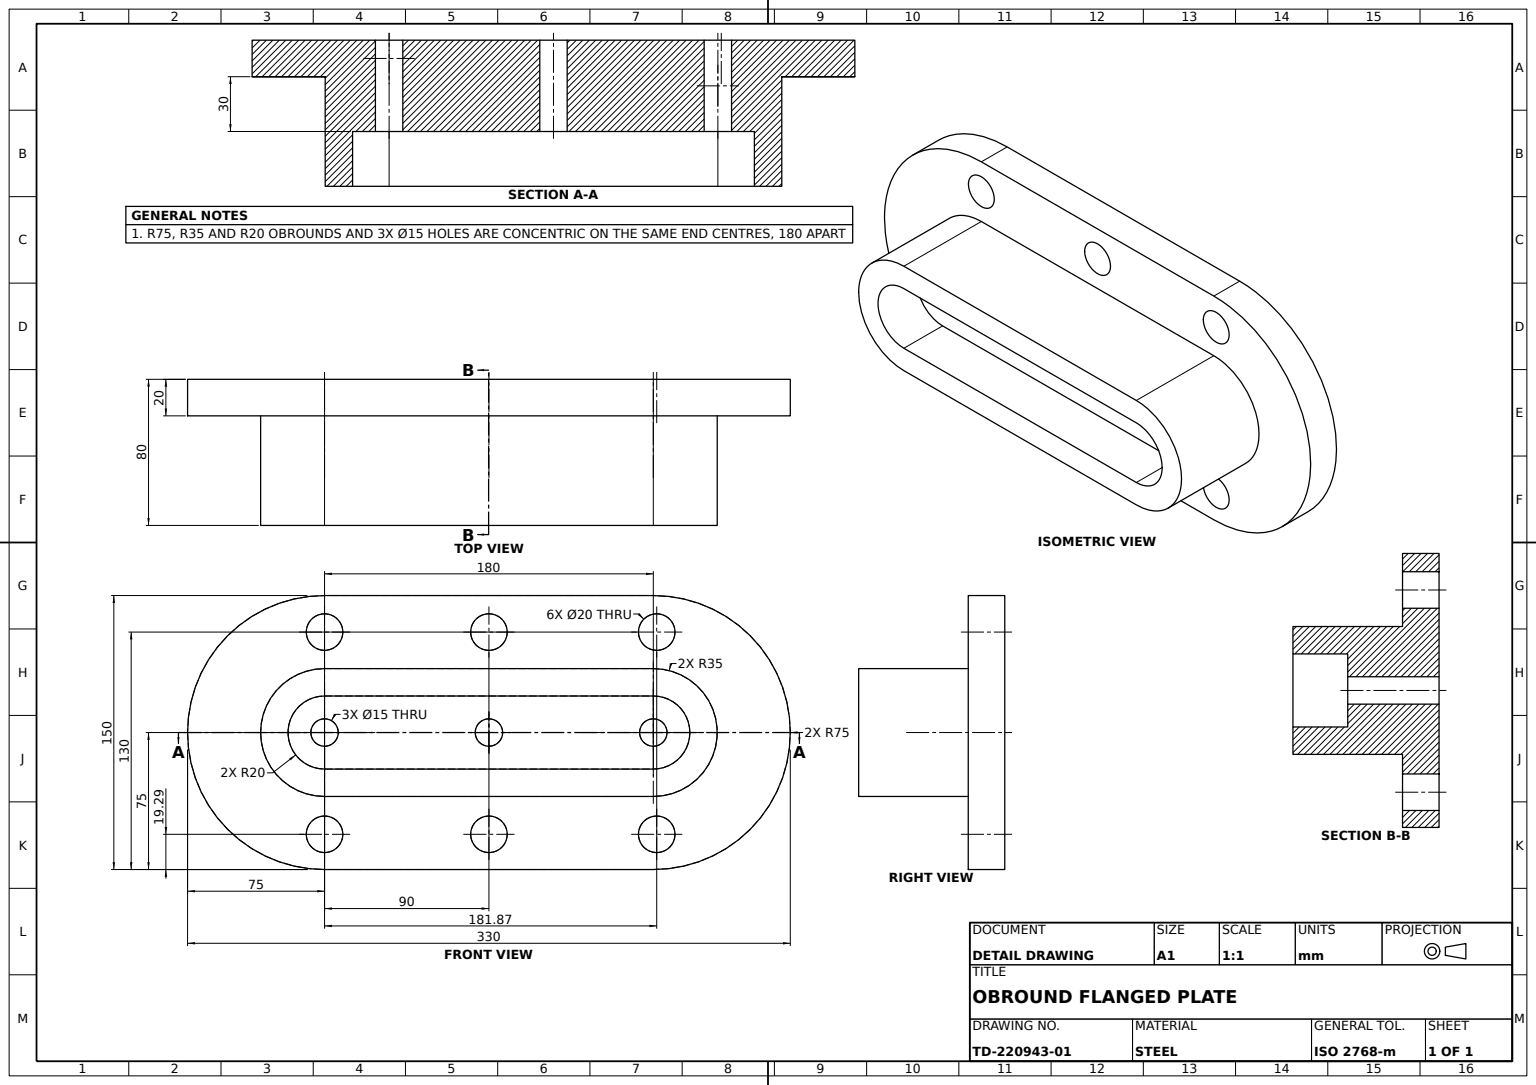
SolidWorks part; units mm, degrees
material "Plain Carbon Steel"
ref_plane "Front Plane" through (0, 0, 0) normal (0, 0, 1) x (1, 0, 0)
ref_plane "Top Plane" through (0, 0, 0) normal (0, 1, 0) x (1, 0, 0)
ref_plane "Right Plane" through (0, 0, 0) normal (1, 0, 0) x (0, 0, -1)
sketch "Flange Plate Sketch" plane through (0, 0, 0) normal (0, 0, 1) x (1, 0, 0)
  line L1 (0, 75) -> (180, 75)
  line L2 (0, -75) -> (180, -75)
  arc A0 (0, 75) -> (0, -75) centre (0, 0) ccw
  arc A1 (180, -75) -> (180, 75) centre (180, 0) ccw
  dimension "D1" = 75
  dimension "D2" = 180
extrude "Flange Plate" add sketch "Flange Plate Sketch" along normal blind 20
sketch "Neck Boss Sketch" plane through (0, 0, 20) normal (0, 0, 1) x (1, 0, 0)
  line L1 (0, 35) -> (180, 35)
  line L2 (0, -35) -> (180, -35)
  arc A0 (0, 35) -> (0, -35) centre (0, 0) ccw
  arc A1 (180, -35) -> (180, 35) centre (180, 0) ccw
  dimension "D1" = 35
  dimension "D2" = 180
extrude "Obround Neck Boss" add sketch "Neck Boss Sketch" along normal blind 60
sketch "Neck Pocket Sketch" plane through (0, 0, 80) normal (0, 0, 1) x (1, 0, 0)
  line L1 (0, 20) -> (180, 20)
  line L2 (0, -20) -> (180, -20)
  arc A0 (0, 20) -> (0, -20) centre (0, 0) ccw
  arc A1 (180, -20) -> (180, 20) centre (180, 0) ccw
  dimension "D1" = 20
  dimension "D2" = 180
extrude "Neck Pocket" cut sketch "Neck Pocket Sketch" against normal blind 30
sketch "Through Opening Sketch" plane through (0, 0, 50) normal (0, 0, 1) x (1, 0, 0)
  circle A0 centre (0, 0) radius 7.5
  circle A1 centre (180, 0) radius 7.5
  circle A2 centre (90, 0) radius 7.5
  dimension "D1" = 15
  dimension "D2" = 15
  dimension "D3" = 15
  dimension "D4" = 15
  dimension "D5" = 90
extrude "Through Opening" cut sketch "Through Opening Sketch" against normal blind 50
sketch "Mounting Holes Sketch" plane through (0, 0, 20) normal (0, 0, 1) x (1, 0, 0)
  line L0 (180, 75) -> (0, 75) construction
  line L1 (0, -35) -> (180, -35) construction
  circle A0 centre (0, 55) radius 10
  circle A1 centre (181.8713, 55) radius 10
  circle A2 centre (181.8713, -55.7131) radius 10
  circle A3 centre (0, -55.7131) radius 10
  circle A4 centre (90, 55) radius 10
  circle A5 centre (90, -55.7131) radius 10
  dimension "D1" = 20
  dimension "D3" = 20
  dimension "D4" = 20
  dimension "D5" = 20
  dimension "D6" = 20
  dimension "D7" = 20
  dimension "D8" = 20
  dimension "D2" = 20
  dimension "D9" = 90
  dimension "D10" = 181.8713
  dimension "D11" = 20.7131
extrude "Mounting Holes" cut sketch "Mounting Holes Sketch" against normal blind 20
